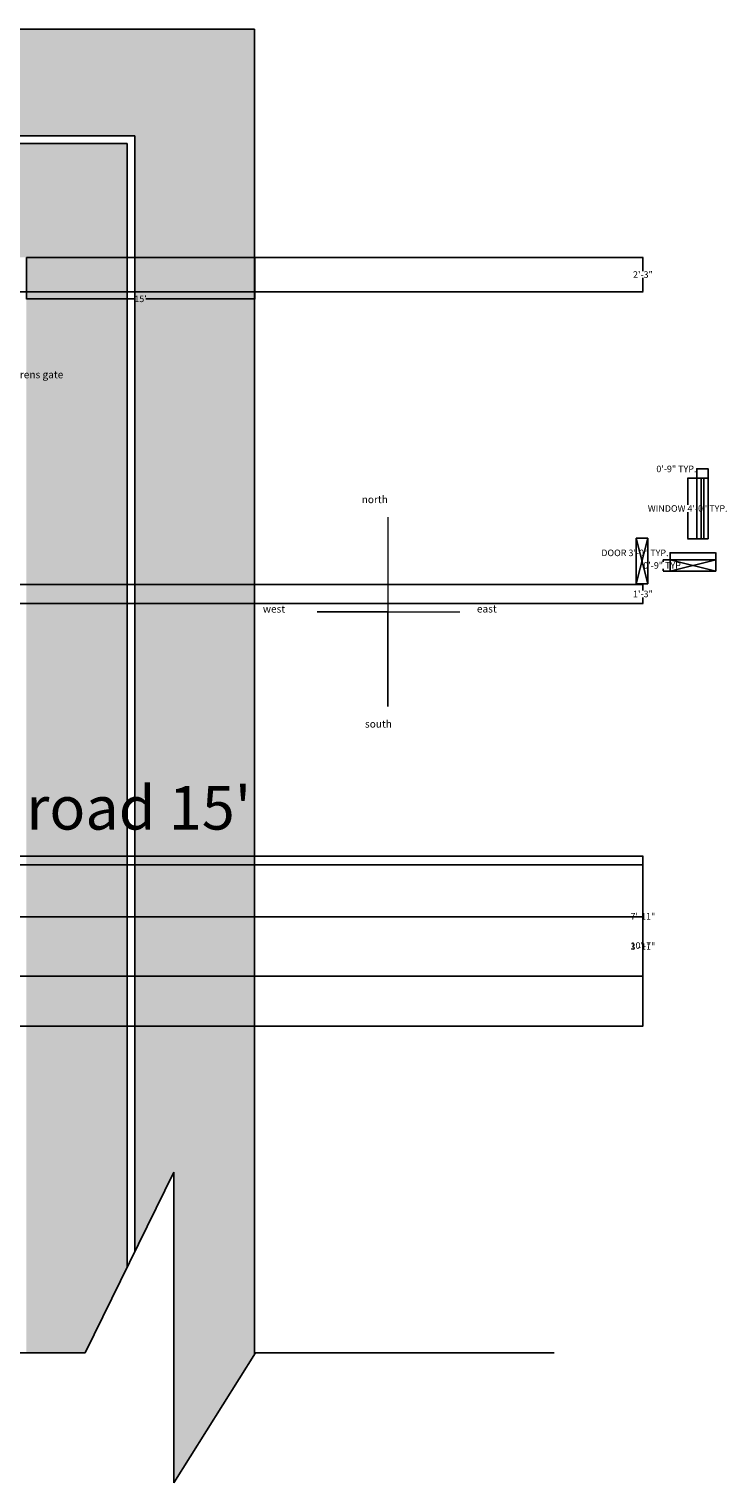
# Model space of a CAD drawing. Units: inches. Extents: x -157 to 1464, y -361 to 1077.
# Tile 9 of 9: x 913 to 1464, y -288 to 859. Entities that reach past the tile are written whole.
import ezdxf

# ---------------------------------------------------------------- set-up
doc = ezdxf.new("R2010")
doc.units = ezdxf.units.IN
doc.header["$MEASUREMENT"] = 0
for name, color, linetype, lineweight in [('A-ANNO-DIMS', 2, 'Continuous', 18), ('A-ANNO-SYMB', 7, 'Continuous', 18), ('A-ANNO-TEXT', 7, 'Continuous', 18), ('C-ANNO-DIMS', 2, 'Continuous', 18), ('C-ANNO-TEXT', 7, 'Continuous', 18), ('C-ROAD', 7, 'Continuous', 25), ('C-ROAD-PATT', 8, 'Continuous', 13), ('doors and windows', 33, 'Continuous', 25)]:
    doc.layers.add(name, color=color, linetype=linetype, lineweight=lineweight)
doc.styles.get("Standard").update_dxf_attribs({"font": 'arial.ttf'})
doc.dimstyles.new('Annotative', dxfattribs={"dimscale": 0, "dimtxt": 5.18, "dimasz": 0.18, "dimexe": 0.18, "dimexo": 0.0625, "dimgap": 0.09, "dimtad": 0, "dimtih": 1, "dimtoh": 1, "dimdec": 0, "dimzin": 0, "dimdsep": 46, "dimlunit": 3, "dimtxsty": 'Standard', "dimcen": 0.09, "dimadec": 0, "dimazin": 0, "dimtfac": 1, "dimtdec": 0, "dimtofl": 0, "dimtmove": 0, "dimatfit": 3, "dimfxl": 1, "dimtolj": 1, "dimtzin": 0, "dimarcsym": 0})

# ---------------------------------------------------------------- blocks, each defined once
blk = doc.blocks.new('*D43')
at = {"layer": 'C-ANNO-DIMS', "color": 0, "lineweight": -2, "transparency": 16777216}
for p, q in [((911.3, 678.8), (911.3, 645.9)), ((1091.3, 678.8), (1091.3, 645.9)), ((911.5, 646.1), (997, 646.1)), ((1091.1, 646.1), (1005.5, 646.1))]:
    blk.add_line(p, q, dxfattribs=at)
at = {"layer": 'C-ANNO-DIMS', "color": 0, "transparency": 16777216}
for points in [[(911.5, 646.1), (911.5, 646), (911.3, 646.1)], [(1091.1, 646.1), (1091.1, 646), (1091.3, 646.1)]]:
    blk.add_solid(points, dxfattribs=at)
at = {"layer": 'Defpoints', "color": 0, "transparency": 16777216}
for p in [(911.3, 678.8), (1091.3, 678.8), (1091.3, 646.1)]:
    blk.add_point(p, dxfattribs=at)
at = {"layer": 'C-ANNO-DIMS', "color": 0, "transparency": 16777216, "insert": (1001.3, 646.1), "char_height": 5.18, "attachment_point": 5}
blk.add_mtext("\\A1;15'", dxfattribs=at)
blk = doc.blocks.new('WIN-48x9')
for p, q in [((9, 48), (0, 48)), ((0, 48), (0, 0)), ((3.5, 48), (3.5, 0)), ((5.5, 48), (5.5, 0)), ((9, 48), (9, 0)), ((9, 0), (0, 0))]:
    blk.add_line(p, q)
blk = doc.blocks.new('DOOR-36x9')
for p, q in [((0, 0), (0, 9)), ((0, 9), (36, 0)), ((36, 9), (0, 0)), ((36, 9), (0, 9)), ((0, 0), (36, 0)), ((36, 0), (36, 9))]:
    blk.add_line(p, q)
blk = doc.blocks.new('*D60')
at = {"layer": 'A-ANNO-DIMS', "color": 0, "lineweight": -2, "transparency": 16777216}
for p, q in [((1439.8, 504.8), (1432.5, 504.8)), ((1432.7, 504.6), (1432.7, 483.6)), ((1432.7, 457), (1432.7, 478)), ((1439.8, 456.8), (1432.5, 456.8))]:
    blk.add_line(p, q, dxfattribs=at)
at = {"layer": 'A-ANNO-DIMS', "color": 0, "transparency": 16777216}
for points in [[(1432.7, 504.6), (1432.7, 504.6), (1432.7, 504.8)], [(1432.7, 457), (1432.7, 457), (1432.7, 456.8)]]:
    blk.add_solid(points, dxfattribs=at)
at = {"layer": 'Defpoints', "color": 0, "transparency": 16777216}
for p in [(1439.9, 504.8), (1432.7, 456.8), (1439.9, 456.8)]:
    blk.add_point(p, dxfattribs=at)
at = {"layer": 'A-ANNO-DIMS', "color": 0, "transparency": 16777216, "insert": (1432.7, 480.8), "char_height": 5.18, "attachment_point": 5}
blk.add_mtext('\\A1;WINDOW 4\'-0" TYP.', dxfattribs=at)
blk = doc.blocks.new('*D61')
at = {"layer": 'A-ANNO-DIMS', "color": 0, "lineweight": -2, "transparency": 16777216}
for p, q in [((1439.9, 512), (1439.7, 512)), ((1439.9, 504.9), (1439.9, 512.2)), ((1448.7, 512), (1440.1, 512)), ((1448.9, 504.9), (1448.9, 512.2))]:
    blk.add_line(p, q, dxfattribs=at)
at = {"layer": 'A-ANNO-DIMS', "color": 0, "transparency": 16777216}
for points in [[(1440.1, 512), (1440.1, 512), (1439.9, 512)], [(1448.7, 512), (1448.7, 512), (1448.9, 512)]]:
    blk.add_solid(points, dxfattribs=at)
at = {"layer": 'Defpoints', "color": 0, "transparency": 16777216}
for p in [(1439.9, 512), (1439.9, 504.8), (1448.9, 504.8)]:
    blk.add_point(p, dxfattribs=at)
at = {"layer": 'A-ANNO-DIMS', "color": 0, "transparency": 16777216, "insert": (1423.8, 512), "char_height": 5.18, "attachment_point": 5}
blk.add_mtext('\\A1;0\'-9" TYP.', dxfattribs=at)
blk = doc.blocks.new('*D62')
at = {"layer": 'A-ANNO-DIMS', "color": 0, "lineweight": -2, "transparency": 16777216}
for p, q in [((1418.9, 445.8), (1418.7, 445.8)), ((1418.9, 440.5), (1418.9, 446)), ((1454.7, 445.8), (1419, 445.8)), ((1454.9, 440.5), (1454.9, 446))]:
    blk.add_line(p, q, dxfattribs=at)
at = {"layer": 'A-ANNO-DIMS', "color": 0, "transparency": 16777216}
for points in [[(1419, 445.8), (1419, 445.8), (1418.9, 445.8)], [(1454.7, 445.8), (1454.7, 445.8), (1454.9, 445.8)]]:
    blk.add_solid(points, dxfattribs=at)
at = {"layer": 'Defpoints', "color": 0, "transparency": 16777216}
for p in [(1418.9, 445.8), (1418.9, 440.4), (1454.9, 440.4)]:
    blk.add_point(p, dxfattribs=at)
at = {"layer": 'A-ANNO-DIMS', "color": 0, "transparency": 16777216, "insert": (1391.1, 445.8), "char_height": 5.18, "attachment_point": 5}
blk.add_mtext('\\A1;DOOR 3\'-0" TYP.', dxfattribs=at)
blk = doc.blocks.new('*D63')
at = {"layer": 'A-ANNO-DIMS', "color": 0, "lineweight": -2, "transparency": 16777216}
for p, q in [((1418.8, 440.4), (1413.3, 440.4)), ((1413.5, 440.2), (1413.5, 438.6)), ((1418.8, 431.4), (1413.3, 431.4)), ((1413.5, 431.6), (1413.5, 433.2))]:
    blk.add_line(p, q, dxfattribs=at)
at = {"layer": 'A-ANNO-DIMS', "color": 0, "transparency": 16777216}
for points in [[(1413.4, 440.2), (1413.5, 440.2), (1413.5, 440.4)], [(1413.4, 431.6), (1413.5, 431.6), (1413.5, 431.4)]]:
    blk.add_solid(points, dxfattribs=at)
at = {"layer": 'Defpoints', "color": 0, "transparency": 16777216}
for p in [(1418.9, 440.4), (1413.5, 431.4), (1418.9, 431.4)]:
    blk.add_point(p, dxfattribs=at)
at = {"layer": 'A-ANNO-DIMS', "color": 0, "transparency": 16777216, "insert": (1413.5, 435.9), "char_height": 5.18, "attachment_point": 5}
blk.add_mtext('\\A1;0\'-9" TYP.', dxfattribs=at)
blk = doc.blocks.new('*D65')
at = {"layer": 'A-ANNO-DIMS', "color": 0, "lineweight": -2, "transparency": 16777216}
for p, q in [((842.5, 199.8), (1397.6, 199.8)), ((1397.4, 199.6), (1397.4, 139)), ((1397.4, 72.8), (1397.4, 133.5)), ((856.6, 72.7), (1397.6, 72.7))]:
    blk.add_line(p, q, dxfattribs=at)
at = {"layer": 'A-ANNO-DIMS', "color": 0, "transparency": 16777216}
for points in [[(1397.4, 199.6), (1397.4, 199.6), (1397.4, 199.8)], [(1397.4, 72.8), (1397.4, 72.8), (1397.4, 72.7)]]:
    blk.add_solid(points, dxfattribs=at)
at = {"layer": 'Defpoints', "color": 0, "transparency": 16777216}
for p in [(842.4, 199.8), (856.6, 72.7), (1397.4, 72.7)]:
    blk.add_point(p, dxfattribs=at)
at = {"layer": 'A-ANNO-DIMS', "color": 0, "transparency": 16777216, "insert": (1397.4, 136.2), "char_height": 5.18, "attachment_point": 5}
blk.add_mtext('\\A1;10\'-7"', dxfattribs=at)
blk = doc.blocks.new('*D68')
at = {"layer": 'A-ANNO-DIMS', "color": 0, "lineweight": -2, "transparency": 16777216}
for p, q in [((911.3, 678.8), (1397.6, 678.8)), ((1397.4, 678.7), (1397.4, 668)), ((1397.4, 651.9), (1397.4, 662.6)), ((862.6, 651.7), (1397.6, 651.7))]:
    blk.add_line(p, q, dxfattribs=at)
at = {"layer": 'A-ANNO-DIMS', "color": 0, "transparency": 16777216}
for points in [[(1397.4, 678.7), (1397.4, 678.7), (1397.4, 678.8)], [(1397.4, 651.9), (1397.4, 651.9), (1397.4, 651.7)]]:
    blk.add_solid(points, dxfattribs=at)
at = {"layer": 'Defpoints', "color": 0, "transparency": 16777216}
for p in [(911.3, 678.8), (1397.4, 678.8), (862.6, 651.7)]:
    blk.add_point(p, dxfattribs=at)
at = {"layer": 'A-ANNO-DIMS', "color": 0, "transparency": 16777216, "insert": (1397.4, 665.3), "char_height": 5.18, "attachment_point": 5}
blk.add_mtext('\\A1;2\'-3"', dxfattribs=at)
blk = doc.blocks.new('*D74')
at = {"layer": 'A-ANNO-DIMS', "color": 0, "lineweight": -2, "transparency": 16777216}
for p, q in [((597, 158.9), (1397.6, 158.9)), ((1397.4, 158.7), (1397.4, 138.1)), ((1397.4, 112), (1397.4, 132.6)), ((597, 111.9), (1397.6, 111.9))]:
    blk.add_line(p, q, dxfattribs=at)
at = {"layer": 'A-ANNO-DIMS', "color": 0, "transparency": 16777216}
for points in [[(1397.4, 158.7), (1397.4, 158.7), (1397.4, 158.9)], [(1397.4, 112), (1397.4, 112), (1397.4, 111.9)]]:
    blk.add_solid(points, dxfattribs=at)
at = {"layer": 'Defpoints', "color": 0, "transparency": 16777216}
for p in [(597, 158.9), (1397.4, 158.9), (597, 111.9)]:
    blk.add_point(p, dxfattribs=at)
at = {"layer": 'A-ANNO-DIMS', "color": 0, "transparency": 16777216, "insert": (1397.4, 135.4), "char_height": 5.18, "attachment_point": 5}
blk.add_mtext('\\A1;3\'-11"', dxfattribs=at)
blk = doc.blocks.new('*D76')
at = {"layer": 'A-ANNO-DIMS', "color": 0, "lineweight": -2, "transparency": 16777216}
for p, q in [((597, 420.9), (1397.6, 420.9)), ((1397.4, 420.7), (1397.4, 416.1)), ((597, 405.9), (1397.6, 405.9)), ((1397.4, 406), (1397.4, 410.6))]:
    blk.add_line(p, q, dxfattribs=at)
at = {"layer": 'A-ANNO-DIMS', "color": 0, "transparency": 16777216}
for points in [[(1397.4, 420.7), (1397.4, 420.7), (1397.4, 420.9)], [(1397.4, 406), (1397.4, 406), (1397.4, 405.9)]]:
    blk.add_solid(points, dxfattribs=at)
at = {"layer": 'Defpoints', "color": 0, "transparency": 16777216}
for p in [(597, 420.9), (1397.4, 420.9), (597, 405.9)]:
    blk.add_point(p, dxfattribs=at)
at = {"layer": 'A-ANNO-DIMS', "color": 0, "transparency": 16777216, "insert": (1397.4, 413.4), "char_height": 5.18, "attachment_point": 5}
blk.add_mtext('\\A1;1\'-3"', dxfattribs=at)
blk = doc.blocks.new('*D83')
at = {"layer": 'A-ANNO-DIMS', "color": 0, "lineweight": -2, "transparency": 16777216}
for p, q in [((652.3, 206.6), (1397.6, 206.6)), ((1397.4, 206.5), (1397.4, 161.9)), ((1397.4, 112), (1397.4, 156.6)), ((597, 111.9), (1397.6, 111.9))]:
    blk.add_line(p, q, dxfattribs=at)
at = {"layer": 'A-ANNO-DIMS', "color": 0, "transparency": 16777216}
for points in [[(1397.4, 206.5), (1397.4, 206.5), (1397.4, 206.6)], [(1397.4, 112), (1397.4, 112), (1397.4, 111.9)]]:
    blk.add_solid(points, dxfattribs=at)
at = {"layer": 'Defpoints', "color": 0, "transparency": 16777216}
for p in [(652.3, 206.6), (1397.4, 206.6), (597, 111.9)]:
    blk.add_point(p, dxfattribs=at)
at = {"layer": 'A-ANNO-DIMS', "color": 0, "transparency": 16777216, "insert": (1397.4, 159.2), "char_height": 5.18, "attachment_point": 5}
blk.add_mtext('\\A1;7\'-11"', dxfattribs=at)

msp = doc.modelspace()

# ---------------------------------------------------------------- hatches: boundary and pattern name
at = {"layer": 'C-ROAD-PATT'}
h = msp.add_hatch(color=256, dxfattribs=at)
h.dxf.hatch_style = 1
h.paths.add_polyline_path([(1091.28, 858.84), (31.23, 858.84), (31.23, 838.38), (161.57, 774.56), (996.76, 774.56), (996.76, -105.32), (1027.51, -42.52), (1027.51, -185.11), (1027.51, -287.61), (1091.28, -186.19)])
h.paths.add_polyline_path([(899.55, 208.71), (1098.57, 208.71), (1098.57, 279.4), (899.55, 279.4)], flags=9)
h = msp.add_hatch(color=256, dxfattribs=at)
h.dxf.hatch_style = 1
h.paths.add_polyline_path([(990.76, 768.56), (31.23, 768.56), (-71.27, 768.56), (31.23, 704.11), (31.23, 678.84), (911.28, 678.84), (911.28, -185.11), (957.69, -185.11), (990.76, -117.57)])
h.paths.add_polyline_path([(899.55, 208.71), (1098.57, 208.71), (1098.57, 279.4), (899.55, 279.4)], flags=9)
h.paths.add_polyline_path([(645.57, 707.88), (844.59, 707.88), (844.59, 778.57), (645.57, 778.57)], flags=9)
h.paths.add_polyline_path([(892.1, 580.27), (940.38, 580.27), (940.38, 592.3), (892.1, 592.3)], flags=25)

# ---------------------------------------------------------------- linework, layer by layer
at = {"layer": 'A-ANNO-SYMB'}
for p, q in [((1196.25, 474), (1196.25, 324.58)), ((1196.25, 399.29), (1140.68, 399.29)), ((1140.68, 399.29), (1252.97, 399.29)), ((1196.25, 324.58), (1196.25, 399.29))]:
    msp.add_line(p, q, dxfattribs=at)
at = {"layer": 'C-ROAD'}
for p, q in [((31.23, 858.84), (1091.28, 858.84)), ((1091.28, 858.84), (1091.28, -186.19)), ((31.23, 768.56), (990.76, 768.56)), ((161.57, 774.56), (996.76, 774.56)), ((990.76, 768.56), (990.76, -117.57)), ((996.76, 774.56), (996.76, -105.32)), ((1027.51, -42.52), (957.69, -185.11)), ((1027.51, -185.11), (1027.51, -42.52)), ((957.69, -185.11), (796.52, -185.11)), ((1027.51, -185.11), (1027.51, -287.61)), ((1027.51, -287.61), (1091.96, -185.11)), ((1327.45, -185.11), (1091.96, -185.11))]:
    msp.add_line(p, q, dxfattribs=at)

# ---------------------------------------------------------------- block references
at = {"layer": 'doors and windows'}
for name, p, rotation in [('WIN-48x9', (1448.91, 504.8), 180), ('DOOR-36x9', (1401.21, 421.28), 89.99999999999996), ('DOOR-36x9', (1454.87, 440.41), 180)]:
    msp.add_blockref(name, p, dxfattribs=dict(at, rotation=rotation))

# ---------------------------------------------------------------- texts
at = {"layer": 'A-ANNO-TEXT', "char_height": 5.84, "attachment_point": 1}
for s, insert in [('north', (1175.67, 490.83)), ('west ', (1097.78, 404.52)), ('east', (1266.51, 404.6)), ('south', (1178.26, 313.83))]:
    msp.add_mtext_dynamic_manual_height_columns(s, width=87.358, gutter_width=29.2, heights=[13.12], dxfattribs=dict(at, insert=insert))
at = {"layer": 'C-ANNO-TEXT', "attachment_point": 1}
for s, width, gutter_width, heights, insert, char_height in [('entrens gate', 87.358, 29.2, [13.12], (893.86, 589.3), 5.8395), ("{\\fArial|b1|i0|c0|p34;road 15'}", 513.204, 171.53, [77.1], (911.28, 261.89), 34.3055)]:
    msp.add_mtext_dynamic_manual_height_columns(s, width=width, gutter_width=gutter_width, heights=heights, dxfattribs=dict(at, insert=insert, char_height=char_height))

# ---------------------------------------------------------------- dimensions: what is measured, and where the dimension line sits
at = {"layer": 'A-ANNO-DIMS'}
for base, p1, p2, picture, middle in [((1397.39, 678.84), (862.57, 651.74), (911.28, 678.84), '*D68', (1397.39, 665.29)), ((1397.39, 420.86), (596.97, 405.86), (596.97, 420.86), '*D76', (1397.39, 413.36)), ((1397.39, 206.63), (596.97, 111.86), (652.25, 206.63), '*D83', (1397.39, 159.25)), ((1397.39, 72.66), (842.44, 199.78), (856.57, 72.66), '*D65', (1397.39, 136.22)), ((1397.39, 158.9), (596.97, 111.86), (596.97, 158.9), '*D74', (1397.39, 135.38))]:
    dim = msp.add_linear_dim(base=base, p1=p1, p2=p2, angle=90, dimstyle='Annotative', override={"dimscale": 1, "dimdec": 1, "dimzin": 1, "dimlunit": 4, "dimfrac": 2}, dxfattribs=at)
    dim.commit()
    dim.dimension.update_dxf_attribs({"geometry": picture, "text_midpoint": middle})
for base, p1, p2, angle, text, picture, middle in [((1439.91, 512), (1448.91, 504.8), (1439.91, 504.8), 180, '<> TYP.', '*D61', (1423.85, 512)), ((1432.71, 456.8), (1439.91, 504.8), (1439.91, 456.8), 270, 'WINDOW <> TYP.', '*D60', (1432.71, 480.8)), ((1418.87, 445.81), (1454.87, 440.41), (1418.87, 440.41), 180, 'DOOR <> TYP.', '*D62', (1391.08, 445.81)), ((1413.47, 431.41), (1418.87, 440.41), (1418.87, 431.41), 270, '<> TYP.', '*D63', (1413.47, 435.91))]:
    dim = msp.add_linear_dim(base=base, p1=p1, p2=p2, angle=angle, text=text, dimstyle='Annotative', override={"dimscale": 1, "dimdec": 1, "dimzin": 1, "dimlunit": 4, "dimfrac": 2}, dxfattribs=at)
    dim.commit()
    dim.dimension.update_dxf_attribs({"geometry": picture, "text_midpoint": middle})
at = {"layer": 'C-ANNO-DIMS'}
dim = msp.add_linear_dim(base=(1091.28, 646.07), p1=(911.28, 678.84), p2=(1091.28, 678.84), dimstyle='Annotative', override={"dimclrd": 0, "dimclre": 0, "dimclrt": 0}, dxfattribs=at)
dim.commit()
dim.dimension.update_dxf_attribs({"geometry": '*D43', "text_midpoint": (1001.28, 646.07)})

doc.saveas('drawing.dxf')
